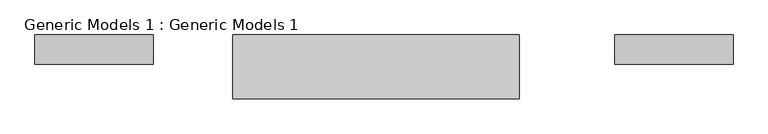
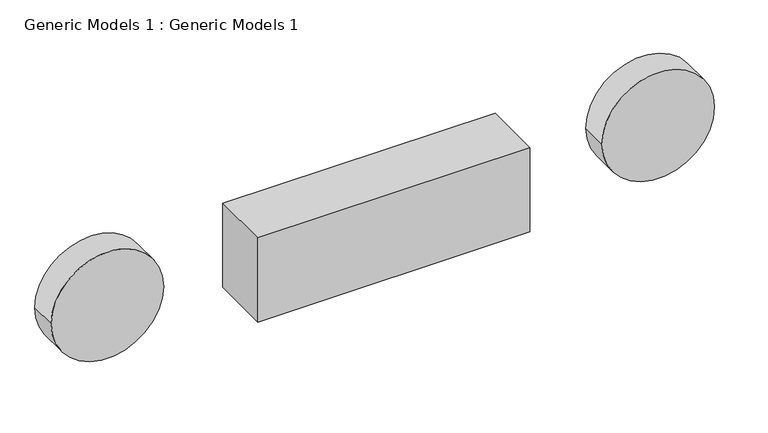
"""IFC4 building model written with IfcOpenShell, lengths in millimetres: proxy geometry, Generic Models 1 : Generic Models 1."""

from ifc_helpers import new_model, si_unit, point, frame, frame_2d, origin, place, context, project, spatial, polyline, circle_curve, trimmed, segment, composite_curve, outline, extrude, source, transform, mapped, element, save


def generic_models_1_generic_models_1_f32fedec(model_context):
    return source(origin(), model_context, "Body", "SweptSolid", [
        extrude(outline(composite_curve([segment(trimmed(circle_curve(frame_2d((10375.8313809, -4360.3915084)), 609.6), [point((10375.8313809, -4969.9915084))], [point((10375.8313809, -3750.7915084))], False, "CARTESIAN"), True, "CONTINUOUS"), segment(trimmed(circle_curve(frame_2d((10375.8313809, -4360.3915084)), 609.6), [point((10375.8313809, -3750.7915084))], [point((10375.8313809, -4969.9915084))], False, "CARTESIAN"), True, "CONTINUOUS")], self_intersect=False)), frame((0.0, -5145.0564015, 0.0), z_axis=(0.0, 1.0, 0.0), x_axis=(0.0, 0.0, 1.0)), (0.0, 0.0, 1.0), 304.8),
        extrude(outline(composite_curve([segment(trimmed(circle_curve(frame_2d((10344.6076896, 1615.1672237)), 609.6), [point((10344.6076896, 1005.5672237))], [point((10344.6076896, 2224.7672237))], False, "CARTESIAN"), True, "CONTINUOUS"), segment(trimmed(circle_curve(frame_2d((10344.6076896, 1615.1672237)), 609.6), [point((10344.6076896, 2224.7672237))], [point((10344.6076896, 1005.5672237))], False, "CARTESIAN"), True, "CONTINUOUS")], self_intersect=False)), frame((0.0, -5145.0564015, 0.0), z_axis=(0.0, 1.0, 0.0), x_axis=(0.0, 0.0, 1.0)), (0.0, 0.0, 1.0), 304.8),
        extrude(outline(polyline([(21.1084916, -5496.4434541), (-2930.038914, -5496.4434541), (-2930.038914, -4840.2564015), (21.1084916, -4840.2564015), (21.1084916, -5496.4434541)])), frame((0.0, 0.0, 9895.1261282), z_axis=(0.0, 0.0, 1.0), x_axis=(1.0, 0.0, 0.0)), (0.0, 0.0, 1.0), 964.4695987),
    ])


if __name__ == "__main__":
    model = new_model("IFC4")
    model_context = context("Model", 3, world=origin())
    ifc_project = project(units=[si_unit("LENGTHUNIT", "METRE", prefix="MILLI")], contexts=[model_context])
    site = spatial("IfcSite", under=ifc_project)
    building = spatial("IfcBuilding", under=site)
    placement = place(None, origin())
    generic_models_1_generic_models_1_shape = generic_models_1_generic_models_1_f32fedec(model_context)
    element("IfcBuildingElementProxy", 1, Name="Generic Models 1 : Generic Models 1", ObjectType="Generic Models 1 : Generic Models 1", at=placement, inside=building, context=model_context, shape_type="MappedRepresentation", body=[
        mapped(generic_models_1_generic_models_1_shape, transform((0.0, 0.0, 0.0), x_axis=(1.0, 0.0, 0.0), y_axis=(0.0, 1.0, 0.0), z_axis=(0.0, 0.0, 1.0))),
    ])
    save(model, "model.ifc")

# Revit data of these elements
# Element 1 (IfcBuildingElementProxy, "Generic Models 1 : Generic Models 1")
#   Materials on its faces: "Parking Stripe", "Brick, Common"
# Materials
#   "Parking Stripe": class "Paint", colour RGB 250 250 91, transparency 0, Cost = 0
#   "Brick, Common": class "Masonry", colour RGB 170 98 104, transparency 0, Description = "Common brick", Cost = 0
